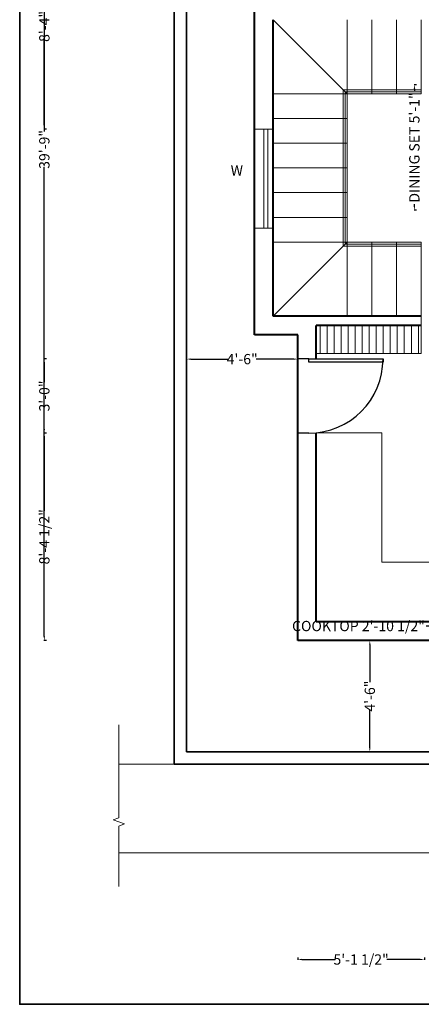
# Model space of a CAD drawing. Units: inches. Extents: x -231 to 349, y -511 to 252.
# Tile 1 of 6: x -231 to -36, y -511 to -33. Entities that reach past the tile are written whole.
import ezdxf

# ---------------------------------------------------------------- set-up
doc = ezdxf.new("R2010")
doc.units = ezdxf.units.IN
doc.header["$MEASUREMENT"] = 0
for name, color, linetype, lineweight in [('A-ANNO-DIMS', 7, 'Continuous', 18), ('A-ANNO-TEXT', 7, 'Continuous', 18), ('A-ANNO-TTLB', 7, 'Continuous', 35), ('A-FLOR-CASE', 30, 'Continuous', 20), ('A-FLOR-PATT', 8, 'Continuous', 13), ('A-FLOR-STRS', 7, 'Continuous', 20), ('A-GLAZ', 177, 'Continuous', 20), ('A-WALL', 7, 'Continuous', 40), ('C-PROP', 7, 'Continuous', 35), ('C-ROAD', 8, 'Continuous', 18), ('DOOR', 42, 'Continuous', 25)]:
    doc.layers.add(name, color=color, linetype=linetype, lineweight=lineweight)
doc.styles.get("Standard").update_dxf_attribs({"font": 'arial.ttf'})
doc.dimstyles.get("Standard").update_dxf_attribs({"dimtxt": 5, "dimasz": 2, "dimexe": 0.18, "dimexo": 0.0625, "dimgap": 0.09, "dimtad": 0, "dimzin": 0, "dimdsep": 46, "dimlunit": 4, "dimtxsty": 'Standard', "dimcen": 0.09, "dimadec": 0, "dimazin": 0, "dimtfac": 1, "dimtofl": 0, "dimtmove": 0, "dimatfit": 3, "dimfxl": 1, "dimfxlon": 1, "dimtolj": 1, "dimtzin": 0, "dimarcsym": 0})

# ---------------------------------------------------------------- blocks, each defined once
blk = doc.blocks.new('*U2')
for p, q in [((0, 0), (0, -6)), ((40, 0), (40, -6))]:
    blk.add_line(p, q)
blk.add_lwpolyline([(0, 0), (0, 40), (1.75, 40), (1.75, 0)], close=True)
blk.add_arc((0, 0), 40, 0, 90)
blk = doc.blocks.new('*D16')
at = {"layer": 'A-ANNO-DIMS', "color": 0, "lineweight": -2, "transparency": 16777216}
for p, q in [((-62.1, -334.62), (-60.92, -334.62)), ((-61.1, -336.62), (-61.1, -354.78)), ((-61.1, -386.62), (-61.1, -368.46)), ((-62.1, -388.62), (-60.92, -388.62))]:
    blk.add_line(p, q, dxfattribs=at)
at = {"layer": 'A-ANNO-DIMS', "color": 0, "transparency": 16777216}
for points in [[(-61.43, -336.62), (-60.76, -336.62), (-61.1, -334.62)], [(-61.43, -386.62), (-60.76, -386.62), (-61.1, -388.62)]]:
    blk.add_solid(points, dxfattribs=at)
at = {"layer": 'Defpoints', "color": 0, "transparency": 16777216}
for p in [(-68.39, -334.62), (-61.1, -334.62), (-68.39, -388.62)]:
    blk.add_point(p, dxfattribs=at)
at = {"layer": 'A-ANNO-DIMS', "color": 0, "transparency": 16777216, "insert": (-61.1, -361.62), "char_height": 5, "attachment_point": 5, "rotation": 90}
blk.add_mtext('\\A1;4\'-6"', dxfattribs=at)
blk = doc.blocks.new('*D17')
at = {"layer": 'A-ANNO-DIMS', "color": 0, "lineweight": -2, "transparency": 16777216}
for p, q in [((-150.08, -196.96), (-150.08, -198.14)), ((-148.08, -197.96), (-129.92, -197.96)), ((-98.08, -197.96), (-116.24, -197.96)), ((-96.08, -196.96), (-96.08, -198.14))]:
    blk.add_line(p, q, dxfattribs=at)
at = {"layer": 'A-ANNO-DIMS', "color": 0, "transparency": 16777216}
for points in [[(-148.08, -197.63), (-148.08, -198.3), (-150.08, -197.96)], [(-98.08, -197.63), (-98.08, -198.3), (-96.08, -197.96)]]:
    blk.add_solid(points, dxfattribs=at)
at = {"layer": 'Defpoints', "color": 0, "transparency": 16777216}
for p in [(-150.08, -194.64), (-96.08, -194.64), (-150.08, -197.96)]:
    blk.add_point(p, dxfattribs=at)
at = {"layer": 'A-ANNO-DIMS', "color": 0, "transparency": 16777216, "insert": (-123.08, -197.96), "char_height": 5, "attachment_point": 5}
blk.add_mtext('\\A1;4\'-6"', dxfattribs=at)
blk = doc.blocks.new('WIN-48IN')
for p, q in [((224.92, -56.7), (233.92, -56.7)), ((227.42, -56.7), (227.42, -104.7)), ((229.42, -56.7), (229.42, -104.7)), ((224.92, -104.7), (233.92, -104.7))]:
    blk.add_line(p, q)
blk = doc.blocks.new('*D38')
at = {"layer": 'A-ANNO-DIMS', "color": 0, "lineweight": -2, "transparency": 16777216}
for p, q in [((-31.7, -327.6), (-33.7, -327.6)), ((-31.7, -326.6), (-31.7, -327.78)), ((0.82, -327.6), (-29.7, -327.6)), ((2.82, -326.6), (2.82, -327.78))]:
    blk.add_line(p, q, dxfattribs=at)
at = {"layer": 'A-ANNO-DIMS', "color": 0, "transparency": 16777216}
for points in [[(-29.7, -327.27), (-29.7, -327.94), (-31.7, -327.6)], [(0.82, -327.27), (0.82, -327.94), (2.82, -327.6)]]:
    blk.add_solid(points, dxfattribs=at)
at = {"layer": 'Defpoints', "color": 0, "transparency": 16777216}
for p in [(-31.7, -322.43), (2.82, -322.43), (-31.7, -327.6)]:
    blk.add_point(p, dxfattribs=at)
at = {"layer": 'A-ANNO-DIMS', "color": 0, "transparency": 16777216, "insert": (-66.61, -327.6), "char_height": 5, "attachment_point": 5}
blk.add_mtext('\\A1;COOKTOP 2\'-10 1/2"', dxfattribs=at)
blk = doc.blocks.new('*D40')
at = {"layer": 'A-ANNO-DIMS', "color": 0, "lineweight": -2, "transparency": 16777216}
for p, q in [((-38.45, -64.68), (-39.63, -64.68)), ((-39.45, -66.68), (-39.45, -67.62)), ((-39.45, -123.69), (-39.45, -122.75)), ((-38.45, -125.69), (-39.63, -125.69))]:
    blk.add_line(p, q, dxfattribs=at)
at = {"layer": 'A-ANNO-DIMS', "color": 0, "transparency": 16777216}
for points in [[(-39.78, -66.68), (-39.12, -66.68), (-39.45, -64.68)], [(-39.78, -123.69), (-39.12, -123.69), (-39.45, -125.69)]]:
    blk.add_solid(points, dxfattribs=at)
at = {"layer": 'Defpoints', "color": 0, "transparency": 16777216}
for p in [(-39.45, -64.68), (-30.3, -64.68), (-30.3, -125.69)]:
    blk.add_point(p, dxfattribs=at)
at = {"layer": 'A-ANNO-DIMS', "color": 0, "transparency": 16777216, "insert": (-39.45, -95.19), "char_height": 5, "attachment_point": 5, "rotation": 90}
blk.add_mtext('\\A1;DINING SET 5\'-1"', dxfattribs=at)
blk = doc.blocks.new('*D47')
at = {"layer": 'A-ANNO-DIMS', "color": 0, "lineweight": -2, "transparency": 16777216}
for p, q in [((-218.19, 142.38), (-219.37, 142.38)), ((-219.19, 140.38), (-219.19, -87.44)), ((-219.19, -332.62), (-219.19, -104.8)), ((-218.19, -334.62), (-219.37, -334.62))]:
    blk.add_line(p, q, dxfattribs=at)
at = {"layer": 'A-ANNO-DIMS', "color": 0, "transparency": 16777216}
for points in [[(-219.53, 140.38), (-218.86, 140.38), (-219.19, 142.38)], [(-219.53, -332.62), (-218.86, -332.62), (-219.19, -334.62)]]:
    blk.add_solid(points, dxfattribs=at)
at = {"layer": 'Defpoints', "color": 0, "transparency": 16777216}
for p in [(-117.08, 142.38), (-219.19, -334.62), (-96.08, -334.62)]:
    blk.add_point(p, dxfattribs=at)
at = {"layer": 'A-ANNO-DIMS', "color": 0, "transparency": 16777216, "insert": (-219.19, -96.12), "char_height": 5, "attachment_point": 5, "rotation": 90}
blk.add_mtext('\\A1;39\'-9"', dxfattribs=at)
blk = doc.blocks.new('*D53')
at = {"layer": 'A-ANNO-DIMS', "color": 0, "lineweight": -2, "transparency": 16777216}
for p, q in [((-218.19, 13.57), (-219.37, 13.57)), ((-219.19, 11.57), (-219.19, -29.65)), ((-219.19, -84.36), (-219.19, -43.13)), ((-218.19, -86.36), (-219.37, -86.36))]:
    blk.add_line(p, q, dxfattribs=at)
at = {"layer": 'A-ANNO-DIMS', "color": 0, "transparency": 16777216}
for points in [[(-219.53, 11.57), (-218.86, 11.57), (-219.19, 13.57)], [(-219.53, -84.36), (-218.86, -84.36), (-219.19, -86.36)]]:
    blk.add_solid(points, dxfattribs=at)
at = {"layer": 'Defpoints', "color": 0, "transparency": 16777216}
for p in [(-117.08, 13.57), (-219.19, -86.36), (-117.08, -86.36)]:
    blk.add_point(p, dxfattribs=at)
at = {"layer": 'A-ANNO-DIMS', "color": 0, "transparency": 16777216, "insert": (-219.19, -36.39), "char_height": 5, "attachment_point": 5, "rotation": 90}
blk.add_mtext('\\A1;8\'-4"', dxfattribs=at)
blk = doc.blocks.new('*D56')
at = {"layer": 'A-ANNO-DIMS', "color": 0, "lineweight": -2, "transparency": 16777216}
for p, q in [((-96.08, -488.55), (-96.08, -489.73)), ((-94.08, -489.55), (-77.89, -489.55)), ((-36.58, -489.55), (-52.77, -489.55)), ((-34.58, -488.55), (-34.58, -489.73))]:
    blk.add_line(p, q, dxfattribs=at)
at = {"layer": 'A-ANNO-DIMS', "color": 0, "transparency": 16777216}
for points in [[(-94.08, -489.21), (-94.08, -489.88), (-96.08, -489.55)], [(-36.58, -489.21), (-36.58, -489.88), (-34.58, -489.55)]]:
    blk.add_solid(points, dxfattribs=at)
at = {"layer": 'Defpoints', "color": 0, "transparency": 16777216}
for p in [(-96.08, -334.62), (-34.58, -334.62), (-34.58, -489.55)]:
    blk.add_point(p, dxfattribs=at)
at = {"layer": 'A-ANNO-DIMS', "color": 0, "transparency": 16777216, "insert": (-65.33, -489.55), "char_height": 5, "attachment_point": 5}
blk.add_mtext('\\A1;5\'-1 1/2"', dxfattribs=at)
blk = doc.blocks.new('*D65')
at = {"layer": 'A-ANNO-DIMS', "color": 0, "lineweight": -2, "transparency": 16777216}
for p, q in [((-218.19, -197.87), (-219.37, -197.87)), ((-219.19, -199.87), (-219.19, -209.14)), ((-219.19, -231.87), (-219.19, -222.61)), ((-218.19, -233.87), (-219.37, -233.87))]:
    blk.add_line(p, q, dxfattribs=at)
at = {"layer": 'A-ANNO-DIMS', "color": 0, "transparency": 16777216}
for points in [[(-219.53, -199.87), (-218.86, -199.87), (-219.19, -197.87)], [(-219.53, -231.87), (-218.86, -231.87), (-219.19, -233.87)]]:
    blk.add_solid(points, dxfattribs=at)
at = {"layer": 'Defpoints', "color": 0, "transparency": 16777216}
for p in [(-96.08, -197.87), (-219.19, -233.87), (-96.08, -233.87)]:
    blk.add_point(p, dxfattribs=at)
at = {"layer": 'A-ANNO-DIMS', "color": 0, "transparency": 16777216, "insert": (-219.19, -215.87), "char_height": 5, "attachment_point": 5, "rotation": 90}
blk.add_mtext('\\A1;3\'-0"', dxfattribs=at)
blk = doc.blocks.new('*D66')
at = {"layer": 'A-ANNO-DIMS', "color": 0, "lineweight": -2, "transparency": 16777216}
for p, q in [((-218.19, -233.87), (-219.37, -233.87)), ((-219.19, -235.87), (-219.19, -271.68)), ((-219.19, -332.62), (-219.19, -296.81)), ((-218.19, -334.62), (-219.37, -334.62))]:
    blk.add_line(p, q, dxfattribs=at)
at = {"layer": 'A-ANNO-DIMS', "color": 0, "transparency": 16777216}
for points in [[(-219.53, -235.87), (-218.86, -235.87), (-219.19, -233.87)], [(-219.53, -332.62), (-218.86, -332.62), (-219.19, -334.62)]]:
    blk.add_solid(points, dxfattribs=at)
at = {"layer": 'Defpoints', "color": 0, "transparency": 16777216}
for p in [(-96.08, -233.87), (-219.19, -334.62), (-96.08, -334.62)]:
    blk.add_point(p, dxfattribs=at)
at = {"layer": 'A-ANNO-DIMS', "color": 0, "transparency": 16777216, "insert": (-219.19, -284.25), "char_height": 5, "attachment_point": 5, "rotation": 90}
blk.add_mtext('\\A1;8\'-4 1/2"', dxfattribs=at)
blk = doc.blocks.new('*D68')
at = {"layer": 'A-ANNO-DIMS', "color": 0, "lineweight": -2, "transparency": 16777216}
for p, q in [((-48.08, 213.78), (-48.08, 214.96)), ((-46.08, 214.78), (-38.08, 214.78)), ((-36.08, 213.78), (-36.08, 214.96)), ((-36.08, 214.78), (-34.08, 214.78))]:
    blk.add_line(p, q, dxfattribs=at)
at = {"layer": 'A-ANNO-DIMS', "color": 0, "transparency": 16777216}
for points in [[(-46.08, 215.11), (-46.08, 214.45), (-48.08, 214.78)], [(-38.08, 215.11), (-38.08, 214.45), (-36.08, 214.78)]]:
    blk.add_solid(points, dxfattribs=at)
at = {"layer": 'Defpoints', "color": 0, "transparency": 16777216}
for p in [(-36.08, 214.78), (-48.08, -177.12), (-36.08, -177.12)]:
    blk.add_point(p, dxfattribs=at)
at = {"layer": 'A-ANNO-DIMS', "color": 0, "transparency": 16777216, "insert": (-27.58, 214.78), "char_height": 5, "attachment_point": 5}
blk.add_mtext('\\A1;1\'-0"', dxfattribs=at)

msp = doc.modelspace()

# ---------------------------------------------------------------- hatches: boundary and pattern name
at = {"layer": 'A-FLOR-PATT'}
h = msp.add_hatch(dxfattribs=at)
h.set_pattern_fill('ANSI31', color=256, scale=27.284, angle=45, style=0)
h.paths.add_polyline_path([(-87.08, -195.176), (-36.08, -195.176), (-36.08, -181.62), (-87.08, -181.62)])

# ---------------------------------------------------------------- linework, layer by layer
at = {"layer": 'A-ANNO-TTLB'}
msp.add_lwpolyline([(-231.158, 252.428), (348.864, 252.428), (348.864, -511.312), (-231.158, -511.312)], close=True, dxfattribs=at)
at = {"layer": 'A-FLOR-CASE'}
for p, q in [((-55.326, -233.694), (-87.08, -233.694)), ((-55.326, -296.522), (-55.326, -233.694)), ((77.92, -296.522), (-55.326, -296.522))]:
    msp.add_line(p, q, dxfattribs=at)
at = {"layer": 'A-FLOR-STRS'}
for p, q in [((-72.08, -69.12), (-108.08, -33.12)), ((-72.08, -69.12), (-72.08, -33.12)), ((-60.08, -69.12), (-60.08, -33.12)), ((-48.08, -69.12), (-48.08, -33.12)), ((-36.08, -69.12), (-36.08, -33.12)), ((-108.08, -69.12), (-72.08, -69.12)), ((-36.08, -67.12), (-74.08, -67.12)), ((-74.08, -67.12), (-74.08, -143.12)), ((-36.08, -68.12), (-73.08, -68.12)), ((-73.08, -68.12), (-73.08, -142.12)), ((-36.08, -69.12), (-72.08, -69.12)), ((-72.08, -69.12), (-72.08, -141.12)), ((-108.08, -81.12), (-72.08, -81.12)), ((-108.08, -93.12), (-72.08, -93.12)), ((-108.08, -105.12), (-72.08, -105.12)), ((-108.08, -117.12), (-72.08, -117.12)), ((-108.08, -129.12), (-72.08, -129.12)), ((-108.08, -135.522), (-108.08, -135.522)), ((-108.08, -141.12), (-72.08, -141.12)), ((-108.08, -177.12), (-72.08, -141.12)), ((-74.08, -143.12), (-36.08, -143.12)), ((-73.08, -142.12), (-36.08, -142.12)), ((-72.08, -141.12), (-72.08, -177.12)), ((-72.08, -141.12), (-36.08, -141.12)), ((-60.08, -141.12), (-60.08, -177.12)), ((-48.08, -141.12), (-48.08, -177.12)), ((-36.08, -141.12), (-36.08, -181.62)), ((-36.08, -195.176), (-36.08, -181.62)), ((-87.08, -195.176), (-36.08, -195.176))]:
    msp.add_line(p, q, dxfattribs=at)
at = {"layer": 'A-WALL'}
for p, q in [((-117.08, -186.12), (-117.08, 142.38)), ((-108.08, -177.12), (-108.08, -33.12)), ((-36.08, -177.12), (-108.08, -177.12)), ((-36.08, -181.62), (-87.08, -181.62)), ((-87.08, -197.875), (-87.08, -181.62)), ((-96.08, -186.12), (-117.08, -186.12)), ((-96.08, -334.62), (-96.08, -186.12)), ((-87.08, -325.62), (-87.08, -233.694)), ((77.92, -325.62), (-87.08, -325.62)), ((86.92, -334.62), (-96.08, -334.62))]:
    msp.add_line(p, q, dxfattribs=at)
at = {"layer": 'C-PROP'}
for p, q in [((-156.08, -394.62), (-156.08, 181.38)), ((-150.08, -388.62), (-150.08, 175.38)), ((68.175, -388.62), (-150.08, -388.62)), ((275.92, -394.62), (-156.08, -394.62))]:
    msp.add_line(p, q, dxfattribs=at)
at = {"layer": 'C-ROAD'}
for p, q in [((-156.08, -394.62), (-183.047, -394.62)), ((298.295, -437.796), (-183.047, -437.796))]:
    msp.add_line(p, q, dxfattribs=at)
msp.add_lwpolyline([(-183.047, -375.528), (-183.047, -420.736), (-185.795, -421.736), (-180.3, -423.736), (-183.047, -424.736), (-183.047, -454.092)], dxfattribs=at)

# ---------------------------------------------------------------- block references
at = {"layer": 'A-GLAZ', "rotation": 180}
msp.add_blockref('WIN-48IN', (116.839, -191.062), dxfattribs=at)
at = {"layer": 'DOOR', "xscale": 0.9, "yscale": 0.9, "zscale": 0.9, "rotation": 270}
msp.add_blockref('*U2', (-90.68, -197.875), dxfattribs=at)

# ---------------------------------------------------------------- texts
at = {"layer": 'A-ANNO-TEXT', "insert": (-128.678, -103.822), "char_height": 5, "attachment_point": 1}
msp.add_mtext_dynamic_manual_height_columns('\\A1;W', width=7.82759, gutter_width=1, heights=[0], dxfattribs=at)

# ---------------------------------------------------------------- dimensions: what is measured, and where the dimension line sits
at = {"layer": 'A-ANNO-DIMS'}
for base, p1, p2, override, picture, middle in [((-36.08, 214.78), (-48.08, -177.12), (-36.08, -177.12), {"dimdec": 1, "dimlfac": 1, "dimrnd": 0, "dimzin": 1, "dimdsep": 46, "dimlunit": 4, "dimfrac": 2}, '*D68', (-27.58, 214.78)), ((-150.08, -197.964), (-96.08, -194.639), (-150.08, -194.639), {"dimclrd": 0, "dimclre": 0, "dimclrt": 0}, '*D17', (-123.08, -197.964)), ((-34.58, -489.548), (-96.08, -334.62), (-34.58, -334.62), {"dimdec": 1, "dimlfac": 1, "dimrnd": 0, "dimzin": 1, "dimdsep": 46, "dimlunit": 4, "dimfrac": 2}, '*D56', (-65.33, -489.548))]:
    dim = msp.add_linear_dim(base=base, p1=p1, p2=p2, dimstyle='Standard', override=override, dxfattribs=at)
    dim.commit()
    dim.dimension.update_dxf_attribs({"geometry": picture, "text_midpoint": middle})
for base, p1, p2, override, picture, middle in [((-219.195, -334.62), (-117.08, 142.38), (-96.08, -334.62), {"dimdec": 1, "dimlfac": 1, "dimrnd": 0, "dimzin": 1, "dimdsep": 46, "dimlunit": 4, "dimfrac": 2}, '*D47', (-219.195, -96.12)), ((-219.195, -86.359), (-117.08, 13.574), (-117.08, -86.359), {"dimdec": 1, "dimlfac": 1, "dimrnd": 0, "dimzin": 1, "dimdsep": 46, "dimlunit": 4, "dimfrac": 2}, '*D53', (-219.195, -36.392)), ((-219.195, -233.875), (-96.08, -197.875), (-96.08, -233.875), {"dimdec": 1, "dimlfac": 1, "dimrnd": 0, "dimzin": 1, "dimdsep": 46, "dimlunit": 4, "dimfrac": 2}, '*D65', (-219.195, -215.875)), ((-219.195, -334.62), (-96.08, -233.875), (-96.08, -334.62), {"dimdec": 1, "dimlfac": 1, "dimrnd": 0, "dimzin": 1, "dimdsep": 46, "dimlunit": 4, "dimfrac": 2}, '*D66', (-219.195, -284.248)), ((-61.096, -334.62), (-68.386, -388.62), (-68.386, -334.62), {"dimclrd": 0, "dimclre": 0, "dimclrt": 0}, '*D16', (-61.096, -361.62))]:
    dim = msp.add_linear_dim(base=base, p1=p1, p2=p2, angle=90, dimstyle='Standard', override=override, dxfattribs=at)
    dim.commit()
    dim.dimension.update_dxf_attribs({"geometry": picture, "text_midpoint": middle})
for base, p1, p2, angle, text, picture, middle in [((-39.449, -64.678), (-30.297, -125.693), (-30.297, -64.678), 90, 'DINING SET <>', '*D40', (-39.449, -95.186)), ((-31.705, -327.604), (2.818, -322.425), (-31.705, -322.425), 180, 'COOKTOP <>', '*D38', (-66.614, -327.604))]:
    dim = msp.add_linear_dim(base=base, p1=p1, p2=p2, angle=angle, text=text, dimstyle='Standard', override={"dimdec": 1, "dimlfac": 1, "dimrnd": 0, "dimzin": 1, "dimdsep": 46, "dimlunit": 4, "dimfrac": 2}, dxfattribs=at)
    dim.commit()
    dim.dimension.update_dxf_attribs({"geometry": picture, "text_midpoint": middle})

doc.saveas('drawing.dxf')
